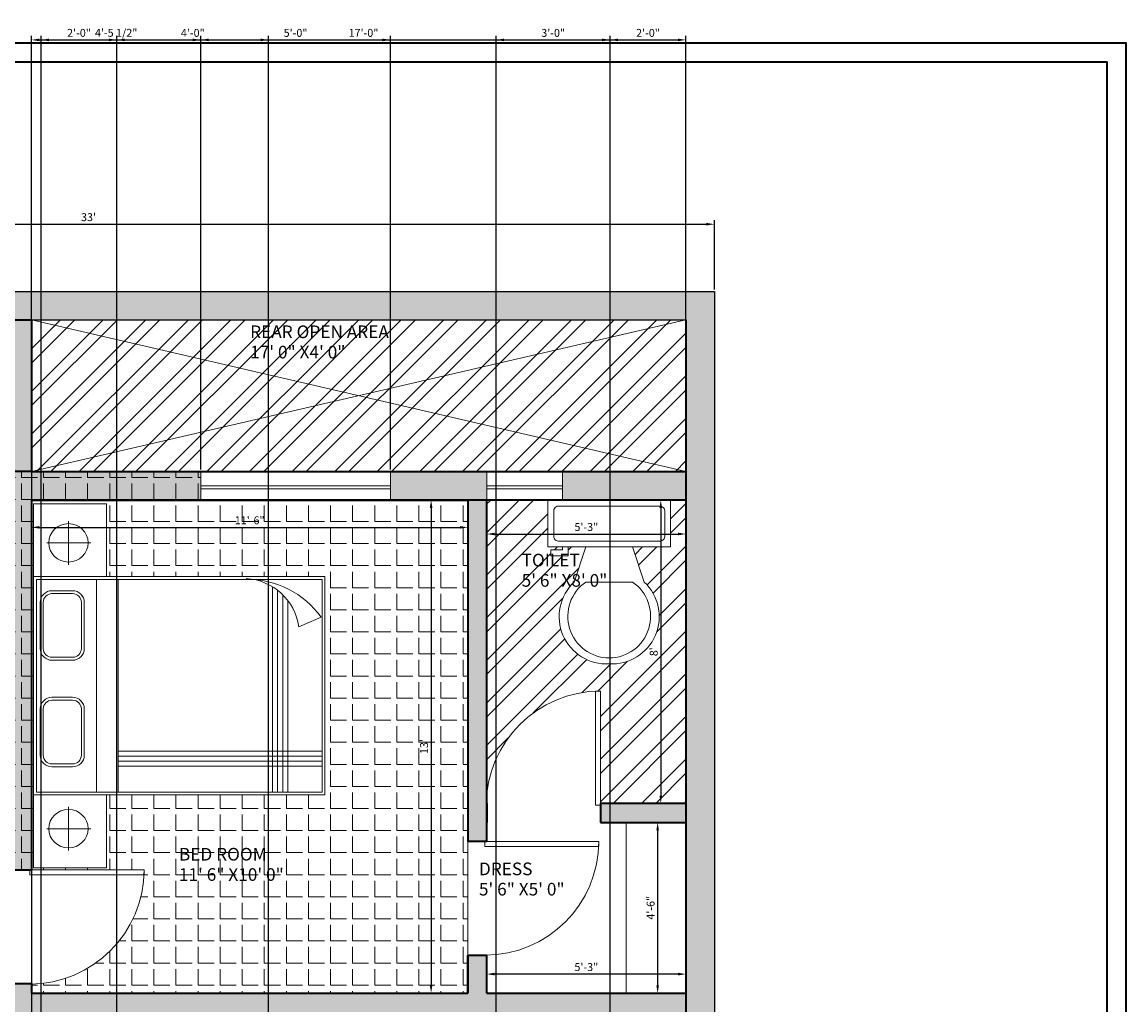
# Model space of a CAD drawing. Units: inches. Extents: x 2004 to 2661, y 1548 to 2351.
# Tile 5 of 5: x 2312 to 2661, y 2040 to 2351. Entities that reach past the tile are written whole.
import ezdxf

# ---------------------------------------------------------------- set-up
doc = ezdxf.new("R2010")
doc.units = ezdxf.units.IN
for name, color, linetype, lineweight in [('A-ANNO-DIMS', 2, 'Continuous', 18), ('A-ANNO-TTLB', 7, 'Continuous', 35), ('A-AREA-IDEN', 7, 'Continuous', 18), ('A-DOOR', 3, 'Continuous', 18), ('A-FLOR-CASE', 8, 'Continuous', 18), ('A-FLOR-FIXT', 9, 'Continuous', 18), ('A-FURN', 8, 'Continuous', 18), ('A-GLAZ', 4, 'Continuous', 18), ('A-SITE', 8, 'Continuous', 13), ('A-WALL', 7, 'Continuous', 35), ('C-PROP', 7, 'Continuous', 25)]:
    doc.layers.add(name, color=color, linetype=linetype, lineweight=lineweight)
doc.layers.add('A-FLOR-PATT', color=18, linetype='Continuous', lineweight=13, true_color=0x000000)
doc.layers.add('A-WALL-PATT', color=18, linetype='Continuous', lineweight=13, true_color=0x000000)
doc.styles.get("Standard").update_dxf_attribs({"font": 'arial.ttf'})
doc.dimstyles.new('Copy of ISO-25', dxfattribs={"dimtxt": 2.5, "dimasz": 2.5, "dimexe": 1.25, "dimexo": 0.625, "dimtad": 1, "dimlunit": 4, "dimtxsty": 'Standard', "dimcen": 2.5, "dimadec": 0, "dimazin": 0, "dimtfac": 1, "dimtmove": 0, "dimatfit": 3, "dimfxl": 1, "dimarcsym": 0})

# ---------------------------------------------------------------- blocks, each defined once
blk = doc.blocks.new('*D1')
at = {"layer": 'A-ANNO-DIMS', "color": 0, "lineweight": -2, "transparency": 16777216}
for p, q in [((2135.26, 2266.72), (2135.26, 2288.6)), ((2137.76, 2287.35), (2528.76, 2287.35)), ((2531.26, 2266.72), (2531.26, 2288.6))]:
    blk.add_line(p, q, dxfattribs=at)
at = {"layer": 'A-ANNO-DIMS', "color": 0, "transparency": 16777216}
for points in [[(2137.76, 2287.77), (2137.76, 2286.93), (2135.26, 2287.35)], [(2528.76, 2287.77), (2528.76, 2286.93), (2531.26, 2287.35)]]:
    blk.add_solid(points, dxfattribs=at)
at = {"layer": 'Defpoints', "color": 0, "transparency": 16777216}
for p in [(2531.26, 2287.35), (2135.26, 2266.09), (2531.26, 2266.09)]:
    blk.add_point(p, dxfattribs=at)
at = {"layer": 'A-ANNO-DIMS', "color": 0, "transparency": 16777216, "insert": (2333.26, 2289.25), "char_height": 2.5, "attachment_point": 5}
blk.add_mtext("33'", dxfattribs=at)
blk = doc.blocks.new('A$C057D194F')
for p, q in [((0, 1.5, -0.1688), (0, 2, -0.1688)), ((0, 2, -0.1688), (0.5, 2, -0.1688)), ((0.5, 2, -0.1688), (0.5, 0, -0.1688)), ((2, 2, -0.1688), (0.5, 2, -0.1688)), ((1.98, 1.98, -0.1688), (0.52, 1.98, -0.1688)), ((0.52, 1.98, -0.1688), (0.52, 0.02, -0.1688)), ((1.98, 0.02, -0.1688), (1.98, 1.98, -0.1688)), ((2, 0, -0.1688), (2, 2, -0.1688)), ((2.5, 2, -0.1688), (2, 2, -0.1688)), ((2.5, 1.5, -0.1688), (2.5, 2, -0.1688)), ((0.2687, 1.9081, -0.1688), (0.2687, 1.761, -0.1688)), ((0.2687, 1.6081, -0.1688), (0.2687, 1.9081, -0.1688)), ((1.0907, 1.9539, -0.1688), (0.7735, 1.9539, -0.1688)), ((1.0907, 1.9339, -0.1688), (0.7735, 1.9339, -0.1688)), ((1.8224, 1.9539, -0.1688), (1.5052, 1.9539, -0.1688)), ((1.8224, 1.9339, -0.1688), (1.5052, 1.9339, -0.1688)), ((2.2313, 1.9081, -0.1688), (2.2313, 1.761, -0.1688)), ((2.2313, 1.6081, -0.1688), (2.2313, 1.9081, -0.1688)), ((0.6935, 1.8739, -0.1688), (0.6935, 1.7322, -0.1688)), ((0.7135, 1.8739, -0.1688), (0.7135, 1.7322, -0.1688)), ((1.1507, 1.7322, -0.1688), (1.1507, 1.8739, -0.1688)), ((1.1707, 1.7322, -0.1688), (1.1707, 1.8739, -0.1688)), ((1.4252, 1.8739, -0.1688), (1.4252, 1.7322, -0.1688)), ((1.4452, 1.8739, -0.1688), (1.4452, 1.7322, -0.1688)), ((1.8824, 1.7322, -0.1688), (1.8824, 1.8739, -0.1688)), ((1.9024, 1.7322, -0.1688), (1.9024, 1.8739, -0.1688)), ((0.4194, 1.761, -0.1688), (0.1194, 1.761, -0.1688)), ((0.2687, 1.761, -0.1688), (0.4194, 1.761, -0.1688)), ((0.2687, 1.761, -0.1688), (0.2687, 1.6081, -0.1688)), ((2.0806, 1.761, -0.1688), (2.3806, 1.761, -0.1688)), ((2.2313, 1.761, -0.1688), (2.0806, 1.761, -0.1688)), ((2.2313, 1.761, -0.1688), (2.2313, 1.6081, -0.1688)), ((0.7735, 1.6722, -0.1688), (1.0907, 1.6722, -0.1688)), ((1.5052, 1.6722, -0.1688), (1.8224, 1.6722, -0.1688)), ((0.7735, 1.6522, -0.1688), (1.0907, 1.6522, -0.1688)), ((1.5052, 1.6522, -0.1688), (1.8224, 1.6522, -0.1688)), ((1.98, 1.5693, -0.1688), (0.52, 1.5693, -0.1688)), ((0.5, 1.5, -0.1688), (0, 1.5, -0.1688)), ((2, 1.5, -0.1688), (2.5, 1.5, -0.1688)), ((1.98, 1.4193, -0.1688), (0.52, 1.4193, -0.1688)), ((0.6969, 0.02, -0.1688), (0.6969, 1.4193, -0.1688)), ((0.7319, 0.02, -0.1688), (0.7319, 1.4193, -0.1688)), ((0.7669, 0.02, -0.1688), (0.7669, 1.4193, -0.1688)), ((0.8019, 0.02, -0.1688), (0.8019, 1.4193, -0.1688)), ((0.52, 0.3595, -0.1688), (1.9292, 0.3595, -0.1688)), ((0.52, 0.3245, -0.1688), (1.905, 0.3245, -0.1688)), ((0.52, 0.2895, -0.1688), (1.8742, 0.2895, -0.1688)), ((0.52, 0.2545, -0.1688), (1.8344, 0.2545, -0.1688)), ((1.6548, 0.1789, -0.1688), (1.7198, 0.0251, -0.1688)), ((0.52, 0.02, -0.1688), (1.98, 0.02, -0.1688)), ((0.5, 0, -0.1688), (2, 0, -0.1688))]:
    blk.add_line(p, q)
for centre, radius, start, end in [((0.7735, 1.8739, -0.1688), 0.08, 90, 180), ((0.7735, 1.8739, -0.1688), 0.06, 90, 180), ((1.0907, 1.8739, -0.1688), 0.08, 0, 90), ((1.0907, 1.8739, -0.1688), 0.06, 0, 90), ((1.5052, 1.8739, -0.1688), 0.08, 90, 180), ((1.5052, 1.8739, -0.1688), 0.06, 90, 180), ((1.8224, 1.8739, -0.1688), 0.08, 0, 90), ((1.8224, 1.8739, -0.1688), 0.06, 0, 90), ((0.7735, 1.7322, -0.1688), 0.08, 180, 270), ((0.7735, 1.7322, -0.1688), 0.06, 180, 270), ((1.0907, 1.7322, -0.1688), 0.08, 270, 0), ((1.0907, 1.7322, -0.1688), 0.06, 270, 0), ((1.5052, 1.7322, -0.1688), 0.08, 180, 270), ((1.5052, 1.7322, -0.1688), 0.06, 180, 270), ((1.8224, 1.7322, -0.1688), 0.08, 270, 0), ((1.8224, 1.7322, -0.1688), 0.06, 270, 0), ((1.5992, 0.5623, -0.1688), 0.3874, 278.2518, 356.6808), ((1.363, 0.5286, -0.1688), 0.6171, 305.32946, 1.04595)]:
    blk.add_arc(centre, radius, start, end)
blk.add_ellipse((0.2687, 1.761, -0.1688), major_axis=(0, -0.1351), ratio=0.975448)
at = {"extrusion": (0, 0, -1)}
blk.add_ellipse((2.2313, 1.761, -0.1688), major_axis=(0, 0.1351), ratio=0.975448, dxfattribs=at)
for p in [(0.2687, 1.761, -0.1688), (2.2313, 1.761, -0.1688)]:
    blk.add_point(p)
blk = doc.blocks.new('*U7')
for p, q in [((-40, 0), (-40, 6)), ((0, 0), (0, 6))]:
    blk.add_line(p, q)
blk.add_lwpolyline([(0, 0), (0, -40), (-1.75, -40), (-1.75, 0)], close=True)
blk.add_arc((0, 0), 40, 180, 270)
blk = doc.blocks.new('*U6')
for p, q in [((0, 0), (0, -6)), ((-40, 0), (-40, -6))]:
    blk.add_line(p, q)
blk.add_lwpolyline([(0, 0), (0, 40), (-1.75, 40), (-1.75, 0)], close=True)
blk.add_arc((0, 0), 40, 90, 180)
blk = doc.blocks.new('*U10')
for p, q in [((241.3, -152.4), (241.3, -50.8)), ((-254, -215.9), (-203.2, -215.9)), ((-254, -241.3), (-254, -215.9)), ((-203.2, -215.9), (-203.2, -203.2)), ((-177.8, -203.2), (-177.8, -241.3)), ((-101.6, -203.2), (-152.4, -355.6)), ((101.6, -203.2), (152.4, -355.6)), ((-177.8, -241.3), (-254, -241.3)), ((101.6, -355.6), (-101.6, -355.6))]:
    blk.add_line(p, q)
blk.add_lwpolyline([(266.7, -203.2), (266.7, 0), (-266.7, 0), (-266.7, -203.2)], close=True)
for points in [[(215.9, -25.4), (-215.9, -25.4)], [(-241.3, -50.8), (-241.3, -152.4)], [(-215.9, -177.8), (215.9, -177.8)]]:
    blk.add_lwpolyline(points)
for centre, radius, start, end in [((-219.075, -47.625), 22.45064, 81.8699, 188.1301), ((219.075, -47.625), 22.45064, 351.8699, 98.1301), ((-219.075, -155.575), 22.45064, 171.869898, 278.1301), ((219.075, -155.575), 22.45064, 261.8699, 8.1301), ((-12.12088, -505.93752), 205.61935, 133.01722, 273.38), ((0.94996, -504.77674), 181.02486, 124.50543, 269.7), ((-0.94742, -504.77674), 181.02486, 270.3, 55.4946), ((12.12342, -505.93752), 205.61935, 266.62, 46.9828)]:
    blk.add_arc(centre, radius, start, end)
blk = doc.blocks.new('*D17')
at = {"layer": 'A-ANNO-DIMS', "color": 0, "lineweight": -2, "transparency": 16777216}
for p, q in [((2315.26, 2199.47), (2315.26, 2190.19)), ((2453.26, 2199.47), (2453.26, 2190.19)), ((2317.76, 2191.44), (2450.76, 2191.44))]:
    blk.add_line(p, q, dxfattribs=at)
at = {"layer": 'A-ANNO-DIMS', "color": 0, "transparency": 16777216}
for points in [[(2317.76, 2191.86), (2317.76, 2191.03), (2315.26, 2191.44)], [(2450.76, 2191.86), (2450.76, 2191.03), (2453.26, 2191.44)]]:
    blk.add_solid(points, dxfattribs=at)
at = {"layer": 'Defpoints', "color": 0, "transparency": 16777216}
for p in [(2315.26, 2200.09), (2453.26, 2200.09), (2453.26, 2191.44)]:
    blk.add_point(p, dxfattribs=at)
at = {"layer": 'A-ANNO-DIMS', "color": 0, "transparency": 16777216, "insert": (2384.26, 2193.34), "char_height": 2.5, "attachment_point": 5}
blk.add_mtext('11\'-6"', dxfattribs=at)
blk = doc.blocks.new('*D18')
at = {"layer": 'A-ANNO-DIMS', "color": 0, "lineweight": -2, "transparency": 16777216}
for p, q in [((2452.63, 2200.09), (2440.4, 2200.09)), ((2441.65, 2197.59), (2441.65, 2046.59)), ((2452.63, 2044.09), (2440.4, 2044.09))]:
    blk.add_line(p, q, dxfattribs=at)
at = {"layer": 'A-ANNO-DIMS', "color": 0, "transparency": 16777216}
for points in [[(2441.23, 2197.59), (2442.06, 2197.59), (2441.65, 2200.09)], [(2441.23, 2046.59), (2442.06, 2046.59), (2441.65, 2044.09)]]:
    blk.add_solid(points, dxfattribs=at)
at = {"layer": 'Defpoints', "color": 0, "transparency": 16777216}
for p in [(2453.26, 2200.09), (2441.65, 2044.09), (2453.26, 2044.09)]:
    blk.add_point(p, dxfattribs=at)
at = {"layer": 'A-ANNO-DIMS', "color": 0, "transparency": 16777216, "insert": (2439.74, 2122.09), "char_height": 2.5, "attachment_point": 5, "rotation": 90}
blk.add_mtext("13'", dxfattribs=at)
blk = doc.blocks.new('*D19')
at = {"layer": 'A-ANNO-DIMS', "color": 0, "lineweight": -2, "transparency": 16777216}
for p, q in [((2459.26, 2199.47), (2459.26, 2188.08)), ((2522.26, 2199.47), (2522.26, 2188.08)), ((2461.76, 2189.33), (2519.76, 2189.33))]:
    blk.add_line(p, q, dxfattribs=at)
at = {"layer": 'A-ANNO-DIMS', "color": 0, "transparency": 16777216}
for points in [[(2461.76, 2189.75), (2461.76, 2188.91), (2459.26, 2189.33)], [(2519.76, 2189.75), (2519.76, 2188.91), (2522.26, 2189.33)]]:
    blk.add_solid(points, dxfattribs=at)
at = {"layer": 'Defpoints', "color": 0, "transparency": 16777216}
for p in [(2459.26, 2200.09), (2522.26, 2200.09), (2522.26, 2189.33)]:
    blk.add_point(p, dxfattribs=at)
at = {"layer": 'A-ANNO-DIMS', "color": 0, "transparency": 16777216, "insert": (2490.76, 2191.23), "char_height": 2.5, "attachment_point": 5}
blk.add_mtext('5\'-3"', dxfattribs=at)
blk = doc.blocks.new('*D20')
at = {"layer": 'A-ANNO-DIMS', "color": 0, "lineweight": -2, "transparency": 16777216}
for p, q in [((2521.63, 2200.09), (2513.05, 2200.09)), ((2514.3, 2197.59), (2514.3, 2106.59)), ((2521.63, 2104.09), (2513.05, 2104.09))]:
    blk.add_line(p, q, dxfattribs=at)
at = {"layer": 'A-ANNO-DIMS', "color": 0, "transparency": 16777216}
for points in [[(2513.89, 2197.59), (2514.72, 2197.59), (2514.3, 2200.09)], [(2513.89, 2106.59), (2514.72, 2106.59), (2514.3, 2104.09)]]:
    blk.add_solid(points, dxfattribs=at)
at = {"layer": 'Defpoints', "color": 0, "transparency": 16777216}
for p in [(2522.26, 2200.09), (2514.3, 2104.09), (2522.26, 2104.09)]:
    blk.add_point(p, dxfattribs=at)
at = {"layer": 'A-ANNO-DIMS', "color": 0, "transparency": 16777216, "insert": (2512.4, 2152.09), "char_height": 2.5, "attachment_point": 5, "rotation": 90}
blk.add_mtext("8'", dxfattribs=at)
blk = doc.blocks.new('*D21')
at = {"layer": 'A-ANNO-DIMS', "color": 0, "lineweight": -2, "transparency": 16777216}
for p, q in [((2459.26, 2044.72), (2459.26, 2051.34)), ((2519.76, 2050.09), (2461.76, 2050.09)), ((2522.26, 2044.72), (2522.26, 2051.34))]:
    blk.add_line(p, q, dxfattribs=at)
at = {"layer": 'A-ANNO-DIMS', "color": 0, "transparency": 16777216}
for points in [[(2461.76, 2050.51), (2461.76, 2049.68), (2459.26, 2050.09)], [(2519.76, 2050.51), (2519.76, 2049.68), (2522.26, 2050.09)]]:
    blk.add_solid(points, dxfattribs=at)
at = {"layer": 'Defpoints', "color": 0, "transparency": 16777216}
for p in [(2459.26, 2050.09), (2459.26, 2044.09), (2522.26, 2044.09)]:
    blk.add_point(p, dxfattribs=at)
at = {"layer": 'A-ANNO-DIMS', "color": 0, "transparency": 16777216, "insert": (2490.76, 2051.99), "char_height": 2.5, "attachment_point": 5}
blk.add_mtext('5\'-3"', dxfattribs=at)
blk = doc.blocks.new('*D22')
at = {"layer": 'A-ANNO-DIMS', "color": 0, "lineweight": -2, "transparency": 16777216}
for p, q in [((2521.63, 2098.09), (2512.06, 2098.09)), ((2513.31, 2095.59), (2513.31, 2046.59)), ((2521.63, 2044.09), (2512.06, 2044.09))]:
    blk.add_line(p, q, dxfattribs=at)
at = {"layer": 'A-ANNO-DIMS', "color": 0, "transparency": 16777216}
for points in [[(2512.89, 2095.59), (2513.73, 2095.59), (2513.31, 2098.09)], [(2512.89, 2046.59), (2513.73, 2046.59), (2513.31, 2044.09)]]:
    blk.add_solid(points, dxfattribs=at)
at = {"layer": 'Defpoints', "color": 0, "transparency": 16777216}
for p in [(2522.26, 2098.09), (2513.31, 2044.09), (2522.26, 2044.09)]:
    blk.add_point(p, dxfattribs=at)
at = {"layer": 'A-ANNO-DIMS', "color": 0, "transparency": 16777216, "insert": (2511.41, 2071.09), "char_height": 2.5, "attachment_point": 5, "rotation": 90}
blk.add_mtext('4\'-6"', dxfattribs=at)
blk = doc.blocks.new('WINDOW-PANE-24IN')
for p, q in [((0, 1), (24, 1)), ((0, 0), (24, 0))]:
    blk.add_line(p, q)
blk = doc.blocks.new('*D41')
at = {"layer": 'A-ANNO-DIMS', "color": 0, "lineweight": -2, "transparency": 16777216}
for p, q in [((2318.26, 1675.72), (2318.26, 2346.91)), ((2522.26, 1675.72), (2522.26, 2346.91)), ((2320.76, 2345.66), (2519.76, 2345.66))]:
    blk.add_line(p, q, dxfattribs=at)
at = {"layer": 'A-ANNO-DIMS', "color": 0, "transparency": 16777216}
for points in [[(2320.76, 2346.07), (2320.76, 2345.24), (2318.26, 2345.66)], [(2519.76, 2346.07), (2519.76, 2345.24), (2522.26, 2345.66)]]:
    blk.add_solid(points, dxfattribs=at)
at = {"layer": 'Defpoints', "color": 0, "transparency": 16777216}
for p in [(2522.26, 2345.66), (2318.26, 1675.09), (2522.26, 1675.09)]:
    blk.add_point(p, dxfattribs=at)
at = {"layer": 'A-ANNO-DIMS', "color": 0, "transparency": 16777216, "insert": (2420.26, 2347.56), "char_height": 2.5, "attachment_point": 5}
blk.add_mtext('17\'-0"', dxfattribs=at)
blk = doc.blocks.new('*D42')
at = {"layer": 'A-ANNO-DIMS', "color": 0, "lineweight": -2, "transparency": 16777216}
for p, q in [((2315.26, 2256.47), (2315.26, 1630.09)), ((2522.26, 2256.47), (2522.26, 1630.09)), ((2317.76, 1631.34), (2519.76, 1631.34))]:
    blk.add_line(p, q, dxfattribs=at)
at = {"layer": 'A-ANNO-DIMS', "color": 0, "transparency": 16777216}
for points in [[(2317.76, 1631.76), (2317.76, 1630.93), (2315.26, 1631.34)], [(2519.76, 1631.76), (2519.76, 1630.93), (2522.26, 1631.34)]]:
    blk.add_solid(points, dxfattribs=at)
at = {"layer": 'Defpoints', "color": 0, "transparency": 16777216}
for p in [(2315.26, 2257.09), (2522.26, 2257.09), (2522.26, 1631.34)]:
    blk.add_point(p, dxfattribs=at)
at = {"layer": 'A-ANNO-DIMS', "color": 0, "transparency": 16777216, "insert": (2418.76, 1633.24), "char_height": 2.5, "attachment_point": 5}
blk.add_mtext('17\'-3"', dxfattribs=at)
blk = doc.blocks.new('*D48')
at = {"layer": 'A-ANNO-DIMS', "color": 0, "lineweight": -2, "transparency": 16777216}
for p, q in [((2315.26, 2209.72), (2315.26, 2346.91)), ((2368.77, 2209.72), (2368.77, 2346.91)), ((2317.76, 2345.66), (2366.27, 2345.66))]:
    blk.add_line(p, q, dxfattribs=at)
at = {"layer": 'A-ANNO-DIMS', "color": 0, "transparency": 16777216}
for points in [[(2317.76, 2346.07), (2317.76, 2345.24), (2315.26, 2345.66)], [(2366.27, 2346.07), (2366.27, 2345.24), (2368.77, 2345.66)]]:
    blk.add_solid(points, dxfattribs=at)
at = {"layer": 'Defpoints', "color": 0, "transparency": 16777216}
for p in [(2368.77, 2345.66), (2315.26, 2209.09), (2368.77, 2209.09)]:
    blk.add_point(p, dxfattribs=at)
at = {"layer": 'A-ANNO-DIMS', "color": 0, "transparency": 16777216, "insert": (2342.01, 2347.58), "char_height": 2.5, "attachment_point": 5}
blk.add_mtext('4\'-5 1/2"', dxfattribs=at)
blk = doc.blocks.new('*D49')
at = {"layer": 'A-ANNO-DIMS', "color": 0, "lineweight": -2, "transparency": 16777216}
for p, q in [((2368.77, 2209.72), (2368.77, 2346.91)), ((2428.77, 2209.72), (2428.77, 2346.91)), ((2371.27, 2345.66), (2426.27, 2345.66))]:
    blk.add_line(p, q, dxfattribs=at)
at = {"layer": 'A-ANNO-DIMS', "color": 0, "transparency": 16777216}
for points in [[(2371.27, 2346.07), (2371.27, 2345.24), (2368.77, 2345.66)], [(2426.27, 2346.07), (2426.27, 2345.24), (2428.77, 2345.66)]]:
    blk.add_solid(points, dxfattribs=at)
at = {"layer": 'Defpoints', "color": 0, "transparency": 16777216}
for p in [(2428.77, 2345.66), (2368.77, 2209.09), (2428.77, 2209.09)]:
    blk.add_point(p, dxfattribs=at)
at = {"layer": 'A-ANNO-DIMS', "color": 0, "transparency": 16777216, "insert": (2398.77, 2347.56), "char_height": 2.5, "attachment_point": 5}
blk.add_mtext('5\'-0"', dxfattribs=at)
blk = doc.blocks.new('*D50')
at = {"layer": 'A-ANNO-DIMS', "color": 0, "lineweight": -2, "transparency": 16777216}
for p, q in [((2318.26, 1762.72), (2318.26, 2346.91)), ((2342.26, 1762.72), (2342.26, 2346.91)), ((2320.76, 2345.66), (2339.76, 2345.66))]:
    blk.add_line(p, q, dxfattribs=at)
at = {"layer": 'A-ANNO-DIMS', "color": 0, "transparency": 16777216}
for points in [[(2320.76, 2346.07), (2320.76, 2345.24), (2318.26, 2345.66)], [(2339.76, 2346.07), (2339.76, 2345.24), (2342.26, 2345.66)]]:
    blk.add_solid(points, dxfattribs=at)
at = {"layer": 'Defpoints', "color": 0, "transparency": 16777216}
for p in [(2342.26, 2345.66), (2318.26, 1762.09), (2342.26, 1762.09)]:
    blk.add_point(p, dxfattribs=at)
at = {"layer": 'A-ANNO-DIMS', "color": 0, "transparency": 16777216, "insert": (2330.26, 2347.56), "char_height": 2.5, "attachment_point": 5}
blk.add_mtext('2\'-0"', dxfattribs=at)
blk = doc.blocks.new('*D51')
at = {"layer": 'A-ANNO-DIMS', "color": 0, "lineweight": -2, "transparency": 16777216}
for p, q in [((2342.26, 1762.72), (2342.26, 2346.91)), ((2390.26, 1762.72), (2390.26, 2346.91)), ((2344.76, 2345.66), (2387.76, 2345.66))]:
    blk.add_line(p, q, dxfattribs=at)
at = {"layer": 'A-ANNO-DIMS', "color": 0, "transparency": 16777216}
for points in [[(2344.76, 2346.07), (2344.76, 2345.24), (2342.26, 2345.66)], [(2387.76, 2346.07), (2387.76, 2345.24), (2390.26, 2345.66)]]:
    blk.add_solid(points, dxfattribs=at)
at = {"layer": 'Defpoints', "color": 0, "transparency": 16777216}
for p in [(2390.26, 2345.66), (2342.26, 1762.09), (2390.26, 1762.09)]:
    blk.add_point(p, dxfattribs=at)
at = {"layer": 'A-ANNO-DIMS', "color": 0, "transparency": 16777216, "insert": (2366.26, 2347.56), "char_height": 2.5, "attachment_point": 5}
blk.add_mtext('4\'-0"', dxfattribs=at)
blk = doc.blocks.new('*D52')
at = {"layer": 'A-ANNO-DIMS', "color": 0, "lineweight": -2, "transparency": 16777216}
for p, q in [((2462.26, 1762.72), (2462.26, 2346.91)), ((2498.26, 1762.72), (2498.26, 2346.91)), ((2464.76, 2345.66), (2495.76, 2345.66))]:
    blk.add_line(p, q, dxfattribs=at)
at = {"layer": 'A-ANNO-DIMS', "color": 0, "transparency": 16777216}
for points in [[(2464.76, 2346.07), (2464.76, 2345.24), (2462.26, 2345.66)], [(2495.76, 2346.07), (2495.76, 2345.24), (2498.26, 2345.66)]]:
    blk.add_solid(points, dxfattribs=at)
at = {"layer": 'Defpoints', "color": 0, "transparency": 16777216}
for p in [(2498.26, 2345.66), (2462.26, 1762.09), (2498.26, 1762.09)]:
    blk.add_point(p, dxfattribs=at)
at = {"layer": 'A-ANNO-DIMS', "color": 0, "transparency": 16777216, "insert": (2480.26, 2347.56), "char_height": 2.5, "attachment_point": 5}
blk.add_mtext('3\'-0"', dxfattribs=at)
blk = doc.blocks.new('*D53')
at = {"layer": 'A-ANNO-DIMS', "color": 0, "lineweight": -2, "transparency": 16777216}
for p, q in [((2498.26, 1762.72), (2498.26, 2346.91)), ((2522.26, 1762.72), (2522.26, 2346.91)), ((2500.76, 2345.66), (2519.76, 2345.66))]:
    blk.add_line(p, q, dxfattribs=at)
at = {"layer": 'A-ANNO-DIMS', "color": 0, "transparency": 16777216}
for points in [[(2500.76, 2346.07), (2500.76, 2345.24), (2498.26, 2345.66)], [(2519.76, 2346.07), (2519.76, 2345.24), (2522.26, 2345.66)]]:
    blk.add_solid(points, dxfattribs=at)
at = {"layer": 'Defpoints', "color": 0, "transparency": 16777216}
for p in [(2522.26, 2345.66), (2498.26, 1762.09), (2522.26, 1762.09)]:
    blk.add_point(p, dxfattribs=at)
at = {"layer": 'A-ANNO-DIMS', "color": 0, "transparency": 16777216, "insert": (2510.26, 2347.56), "char_height": 2.5, "attachment_point": 5}
blk.add_mtext('2\'-0"', dxfattribs=at)

msp = doc.modelspace()

# ---------------------------------------------------------------- hatches: boundary and pattern name
at = {"layer": 'A-FLOR-PATT'}
h = msp.add_hatch(dxfattribs=at)
h.set_pattern_fill('ANSI32', color=256)
h.paths.add_polyline_path([(2522.257, 2257.093), (2466.833, 2257.093), (2315.257, 2257.093), (2418.757, 2233.093)])
h.paths.add_polyline_path([(2418.757, 2233.093), (2315.257, 2257.093), (2315.257, 2209.093)])
h.paths.add_polyline_path([(2418.757, 2233.093), (2315.257, 2209.093), (2522.257, 2209.093)])
h.paths.add_polyline_path([(2522.257, 2257.093), (2418.757, 2233.093), (2522.257, 2209.093)])
h.paths.add_polyline_path([(2522.257, 1753.093), (2318.257, 1753.093), (2318.257, 1675.093), (2522.257, 1675.093)])
h.paths.add_polyline_path([(2210.267, 2081.517), (2210.233, 2081.517), (2210.233, 2083.093), (2246.257, 2083.093), (2246.257, 2119.093), (2144.257, 2119.093), (2144.257, 2047.093), (2244.938, 2047.093, -0.390864)])
h.paths.add_polyline_path([(2171.613, 2077.721), (2161.069, 2080.96), (2161.193, 2075.729), (2163.808, 2075.791), (2163.932, 2070.56), (2162.189, 2070.519), (2162.106, 2074.006), (2161.234, 2073.986), (2161.338, 2069.627), (2147.389, 2069.296), (2146.521, 2105.911), (2160.469, 2106.241), (2160.738, 2094.908), (2171.117, 2098.643, -0.7025712), (2195.775, 2088.761, -0.7025621)], flags=16)
h.paths.add_polyline_path([(2171.53, 2081.208), (2171.2, 2095.156, -0.7345333), (2194.031, 2088.72, -0.7345297)], flags=0)
h.paths.add_polyline_path([(2158.245, 2071.298), (2150.835, 2071.122, -0.4142136), (2149.061, 2072.388), (2148.347, 2102.465, -0.4142136), (2149.614, 2104.239), (2157.024, 2104.415, -0.4142136), (2158.798, 2103.149), (2159.512, 2073.072, -0.4142136)], flags=0)
h.paths.add_polyline_path([(2522.257, 2200.093), (2517.397, 2200.093), (2517.397, 2185.232), (2505.384, 2185.232), (2509.08, 2174.143, -0.7025712), (2497.991, 2148.268, -0.7025621), (2486.902, 2174.142), (2490.599, 2185.232), (2485.054, 2185.232), (2485.054, 2182.459), (2479.509, 2182.459), (2479.509, 2184.307), (2483.206, 2184.307), (2483.206, 2185.232), (2478.585, 2185.232), (2478.585, 2200.093), (2459.257, 2200.093), (2459.257, 2106.686, -0.3761573), (2493.676, 2139.619), (2493.676, 2139.653), (2495.257, 2139.653), (2495.257, 2104.093), (2522.257, 2104.093)])
h.paths.add_polyline_path([(2349.854, 1719.146), (2381.921, 1719.146), (2381.921, 1725.273), (2349.854, 1725.273)], flags=24)
h.paths.add_polyline_path([(2349.84, 1725.558), (2388.851, 1725.558), (2388.851, 1731.767), (2349.84, 1731.767)], flags=24)
h.paths.add_polyline_path([(2152.908, 2086.679), (2181.867, 2086.679), (2181.867, 2092.806), (2152.908, 2092.806)], flags=8)
h.paths.add_polyline_path([(2152.895, 2093.091), (2174.525, 2093.091), (2174.525, 2099.3), (2152.895, 2099.3)], flags=8)
h.paths.add_polyline_path([(2515.001, 2150.174), (2515.001, 2154.033), (2509.85, 2154.033), (2509.85, 2150.174)], flags=24)
h.paths.add_polyline_path([(2469.272, 2171.563), (2498.231, 2171.563), (2498.231, 2177.69), (2469.272, 2177.69)], flags=24)
h.paths.add_polyline_path([(2469.258, 2177.975), (2490.888, 2177.975), (2490.888, 2184.184), (2469.258, 2184.184)], flags=24)
h = msp.add_hatch(dxfattribs=at)
h.set_pattern_fill('ANGLE', color=256)
h.set_pattern_definition([(0, (0, 0), (0, 6.985), [5.08, -1.905]), (90, (0, 0), (-6.985, 4e-16), [5.08, -1.905])])
h.paths.add_polyline_path([(2453.257, 2092.093), (2453.257, 2200.093), (2368.773, 2200.093), (2368.773, 2209.093), (2315.257, 2209.093), (2309.257, 2209.093), (2309.257, 2119.093), (2309.257, 2083.093), (2315.257, 2083.093), (2350.837, 2083.093), (2350.837, 2081.511), (2350.802, 2081.511, -0.3968312), (2315.257, 2046.941), (2315.257, 2044.093), (2453.257, 2044.093), (2453.257, 2056.093)])
h.paths.add_polyline_path([(2338.94, 2106.763), (2338.94, 2083.722), (2315.9, 2083.722), (2315.9, 2106.763), (2315.9, 2175.884), (2315.9, 2198.924), (2338.94, 2198.924), (2338.94, 2175.884), (2408.062, 2175.884), (2408.062, 2106.763)], flags=16)
h.paths.add_polyline_path([(2316.822, 2107.684), (2316.822, 2174.962), (2383.185, 2174.962, -0.0091279), (2384.223, 2174.962), (2407.14, 2174.962), (2407.14, 2107.684)], flags=0)
h.paths.add_polyline_path([(2342.657, 2115.838), (2342.657, 2120.677), (2391.497, 2120.677), (2391.497, 2172.623, -0.0921038), (2396.336, 2168.251), (2396.336, 2115.838)], flags=0)
h.paths.add_polyline_path([(2393.11, 2119.064), (2394.723, 2119.064), (2394.723, 2117.451), (2393.11, 2117.451)], flags=0)
edge = h.paths.add_edge_path(flags=0)
edge.add_ellipse((2326.912, 2096.106), major_axis=(-6.224, 0), ratio=0.9754478, start_angle=450, end_angle=540, ccw=False)
edge.add_ellipse((2326.912, 2096.106), major_axis=(-6.224, 0), ratio=0.9754478, start_angle=360, end_angle=450, ccw=False)
edge.add_ellipse((2326.912, 2096.106), major_axis=(-6.224, 0), ratio=0.9754478, start_angle=270, end_angle=360, ccw=False)
edge.add_ellipse((2326.912, 2096.106), major_axis=(-6.224, 0), ratio=0.9754478, start_angle=180, end_angle=270, ccw=False)
h.paths.add_polyline_path([(2328.241, 2115.678), (2321.709, 2115.678, -0.4142136), (2318.023, 2119.364), (2318.023, 2133.984, -0.4142136), (2321.709, 2137.671), (2328.241, 2137.671, -0.4142136), (2331.928, 2133.984), (2331.928, 2119.364, -0.4142136)], flags=0)
h.paths.add_polyline_path([(2328.241, 2116.599), (2321.709, 2116.599, -0.4142136), (2318.945, 2119.364), (2318.945, 2133.984, -0.4142136), (2321.709, 2136.749), (2328.241, 2136.749, -0.4142136), (2331.006, 2133.984), (2331.006, 2119.364, -0.4142136)], flags=0)
h.paths.add_polyline_path([(2328.241, 2149.395), (2321.709, 2149.395, -0.4142136), (2318.023, 2153.081), (2318.023, 2167.701, -0.4142136), (2321.709, 2171.388), (2328.241, 2171.388, -0.4142136), (2331.928, 2167.701), (2331.928, 2153.081, -0.4142136)], flags=0)
h.paths.add_polyline_path([(2328.241, 2150.316), (2321.709, 2150.316, -0.4142136), (2318.945, 2153.081), (2318.945, 2167.701, -0.4142136), (2321.709, 2170.466), (2328.241, 2170.466, -0.4142136), (2331.006, 2167.701), (2331.006, 2153.081, -0.4142136)], flags=0)
edge = h.paths.add_edge_path(flags=0)
edge.add_ellipse((2326.912, 2186.54), major_axis=(-6.224, 0), ratio=0.9754478, start_angle=0, end_angle=90, ccw=False)
edge.add_ellipse((2326.912, 2186.54), major_axis=(-6.224, 0), ratio=0.9754478, start_angle=270, end_angle=360, ccw=False)
edge.add_ellipse((2326.912, 2186.54), major_axis=(-6.224, 0), ratio=0.9754478, start_angle=180, end_angle=270, ccw=False)
edge.add_ellipse((2326.912, 2186.54), major_axis=(-6.224, 0), ratio=0.9754478, start_angle=90, end_angle=180, ccw=False)
h.paths.add_polyline_path([(2309.257, 2209.093), (2309.257, 2257.093), (2144.257, 2257.093), (2144.257, 2137.093), (2257.19, 2137.093), (2257.19, 2125.093), (2273.257, 2125.093), (2273.257, 2119.093), (2309.257, 2119.093)])
h.paths.add_polyline_path([(2183.028, 2229.908), (2159.988, 2229.908), (2159.988, 2252.949), (2183.028, 2252.949), (2252.149, 2252.949), (2275.19, 2252.949), (2275.19, 2229.908), (2252.149, 2229.908), (2252.149, 2160.787), (2183.028, 2160.787)], flags=16)
h.paths.add_polyline_path([(2183.95, 2252.027), (2251.228, 2252.027), (2251.228, 2185.663, -0.0091279), (2251.228, 2184.625), (2251.228, 2161.709), (2183.95, 2161.709)], flags=0)
h.paths.add_polyline_path([(2192.104, 2172.513), (2192.104, 2226.192), (2196.942, 2226.192), (2196.942, 2177.351), (2248.888, 2177.351, -0.0921038), (2244.517, 2172.513)], flags=0)
h.paths.add_polyline_path([(2193.716, 2174.125), (2193.716, 2175.738), (2195.329, 2175.738), (2195.329, 2174.125)], flags=0)
edge = h.paths.add_edge_path(flags=0)
edge.add_ellipse((2172.372, 2241.936), major_axis=(0, 6.224), ratio=0.9754478, start_angle=450, end_angle=540, ccw=False)
edge.add_ellipse((2172.372, 2241.936), major_axis=(0, 6.224), ratio=0.9754478, start_angle=360, end_angle=450, ccw=False)
edge.add_ellipse((2172.372, 2241.936), major_axis=(0, 6.224), ratio=0.9754478, start_angle=270, end_angle=360, ccw=False)
edge.add_ellipse((2172.372, 2241.936), major_axis=(0, 6.224), ratio=0.9754478, start_angle=180, end_angle=270, ccw=False)
h.paths.add_polyline_path([(2191.943, 2240.607), (2191.943, 2247.139, -0.4142136), (2195.63, 2250.826), (2210.25, 2250.826, -0.4142136), (2213.936, 2247.139), (2213.936, 2240.607, -0.4142136), (2210.25, 2236.921), (2195.63, 2236.921, -0.4142136)], flags=0)
h.paths.add_polyline_path([(2192.865, 2240.607), (2192.865, 2247.139, -0.4142136), (2195.63, 2249.904), (2210.25, 2249.904, -0.4142136), (2213.015, 2247.139), (2213.015, 2240.607, -0.4142136), (2210.25, 2237.842), (2195.63, 2237.842, -0.4142136)], flags=0)
h.paths.add_polyline_path([(2225.66, 2240.607), (2225.66, 2247.139, -0.4142136), (2229.347, 2250.826), (2243.967, 2250.826, -0.4142136), (2247.653, 2247.139), (2247.653, 2240.607, -0.4142136), (2243.967, 2236.921), (2229.347, 2236.921, -0.4142136)], flags=0)
h.paths.add_polyline_path([(2226.582, 2240.607), (2226.582, 2247.139, -0.4142136), (2229.347, 2249.904), (2243.967, 2249.904, -0.4142136), (2246.732, 2247.139), (2246.732, 2240.607, -0.4142136), (2243.967, 2237.842), (2229.347, 2237.842, -0.4142136)], flags=0)
edge = h.paths.add_edge_path(flags=0)
edge.add_ellipse((2262.806, 2241.936), major_axis=(0, 6.224), ratio=0.9754478, start_angle=90, end_angle=180, ccw=False)
edge.add_ellipse((2262.806, 2241.936), major_axis=(0, 6.224), ratio=0.9754478, start_angle=0, end_angle=90, ccw=False)
edge.add_ellipse((2262.806, 2241.936), major_axis=(0, 6.224), ratio=0.9754478, start_angle=270, end_angle=360, ccw=False)
edge.add_ellipse((2262.806, 2241.936), major_axis=(0, 6.224), ratio=0.9754478, start_angle=180, end_angle=270, ccw=False)
at = {"layer": 'A-WALL-PATT'}
h = msp.add_hatch(color=256, dxfattribs=at)
h.dxf.hatch_style = 1
h.paths.add_polyline_path([(2315.257, 2266.093), (2135.257, 2266.093), (2135.257, 1666.093), (2531.257, 1666.093), (2531.257, 1753.093), (2522.257, 1753.093), (2522.257, 1675.093), (2144.257, 1675.093), (2144.257, 2038.093), (2180.257, 2038.093), (2180.257, 2047.093), (2144.257, 2047.093), (2144.257, 2257.093), (2309.257, 2257.093), (2315.257, 2257.093)])
h.paths.add_polyline_path([(2522.257, 2266.093), (2315.257, 2266.093), (2315.257, 2257.093), (2522.257, 2257.093)], flags=17)
h.paths.add_polyline_path([(2368.773, 2209.093), (2315.257, 2209.093), (2309.257, 2209.093), (2309.257, 2119.093), (2309.257, 2083.093), (2315.257, 2083.093), (2315.257, 2119.093), (2315.257, 2200.093), (2368.773, 2200.093)], flags=17)
h.paths.add_polyline_path([(2459.257, 2209.093), (2428.773, 2209.093), (2428.773, 2200.093), (2453.257, 2200.093), (2459.257, 2200.093)], flags=17)
h.paths.add_polyline_path([(2522.257, 2209.093), (2483.257, 2209.093), (2483.257, 2200.093), (2522.257, 2200.093)], flags=17)
h.paths.add_polyline_path([(2522.257, 2044.093), (2459.257, 2044.093), (2459.257, 2056.073, -0.004139), (2458.66, 2056.069), (2453.257, 2056.069), (2453.257, 2044.093), (2315.257, 2044.093), (2315.257, 2046.941, -0.0039864), (2314.68, 2046.936), (2309.257, 2046.936), (2309.257, 2038.093), (2315.257, 2038.093), (2522.257, 2038.093)], flags=17)
h.paths.add_polyline_path([(2531.257, 2266.093), (2522.257, 2266.093), (2522.257, 2257.093), (2522.257, 2209.093), (2522.257, 2200.093), (2522.257, 2104.093), (2522.257, 1762.093), (2498.257, 1762.093), (2498.257, 1753.093), (2522.257, 1753.093), (2531.257, 1753.093)], flags=17)
h.paths.add_polyline_path([(2522.257, 2104.093), (2495.257, 2104.093), (2495.257, 2103.514), (2495.257, 2098.093), (2503.401, 2098.093), (2522.257, 2098.093)], flags=17)
h.paths.add_polyline_path([(2455.748, 2073.874), (2484.708, 2073.874), (2484.708, 2080.001), (2455.748, 2080.001)], flags=25)
h.paths.add_polyline_path([(2455.735, 2080.287), (2477.056, 2080.287), (2477.056, 2086.492), (2455.735, 2086.492)], flags=25)
h.paths.add_polyline_path([(2469.272, 2171.563), (2498.231, 2171.563), (2498.231, 2177.69), (2469.272, 2177.69)], flags=25)
h.paths.add_polyline_path([(2469.258, 2177.975), (2490.888, 2177.975), (2490.888, 2184.184), (2469.258, 2184.184)], flags=25)
h.paths.add_polyline_path([(2360.849, 2078.511), (2396.023, 2078.511), (2396.023, 2084.638), (2360.849, 2084.638)], flags=25)
h.paths.add_polyline_path([(2360.835, 2084.923), (2394.883, 2084.923), (2394.883, 2091.132), (2360.835, 2091.132)], flags=25)
h = msp.add_hatch(color=256, dxfattribs=at)
h.dxf.hatch_style = 1
h.paths.add_polyline_path([(2252.257, 2038.093), (2252.257, 2047.093), (2246.257, 2047.093), (2204.257, 2047.093), (2204.257, 2038.093), (2243.257, 2038.093), (2243.257, 1888.093), (2243.257, 1879.093), (2273.257, 1879.093), (2273.257, 1888.093), (2252.257, 1888.093)])
h.paths.add_polyline_path([(2273.257, 2125.093), (2144.257, 2125.093), (2144.257, 2119.093), (2246.257, 2119.093), (2273.257, 2119.093)])
h.paths.add_polyline_path([(2459.257, 2200.093), (2453.257, 2200.093), (2453.257, 2092.093), (2459.257, 2092.093)])
h.paths.add_polyline_path([(2522.257, 1888.093), (2426.257, 1888.093), (2426.257, 1882.093), (2522.257, 1882.093)])
h.paths.add_polyline_path([(2460.257, 1834.093), (2454.257, 1834.093), (2454.257, 1762.093), (2460.257, 1762.093)])
h.paths.add_polyline_path([(2460.257, 1882.093), (2454.257, 1882.093), (2454.257, 1870.093), (2460.257, 1870.093)])
h.paths.add_polyline_path([(2462.257, 1762.093), (2460.257, 1762.093), (2454.257, 1762.093), (2390.257, 1762.093), (2390.257, 1753.093), (2462.257, 1753.093)])
h.paths.add_polyline_path([(2342.257, 1762.093), (2318.257, 1762.093), (2318.257, 1882.093), (2318.257, 1888.093), (2309.257, 1888.093), (2309.257, 1879.093), (2309.257, 1753.093), (2318.257, 1753.093), (2342.257, 1753.093)])
h.paths.add_polyline_path([(2354.257, 1888.093), (2318.257, 1888.093), (2318.257, 1882.093), (2354.257, 1882.093)])
h.paths.add_polyline_path([(2318.257, 1753.093), (2309.257, 1753.093), (2309.257, 1675.093), (2318.257, 1675.093)])
h.paths.add_polyline_path([(2207.257, 1884.43), (2207.257, 1888.093), (2183.257, 1888.093), (2183.257, 1879.093), (2207.257, 1879.093)])
h.paths.add_polyline_path([(2252.257, 2119.093), (2246.257, 2119.093), (2246.257, 2083.093), (2251.66, 2083.093), (2252.257, 2083.093)])
h.paths.add_polyline_path([(2315.257, 2257.093), (2309.257, 2257.093), (2309.257, 2209.093), (2315.257, 2209.093)])

# ---------------------------------------------------------------- linework, layer by layer
at = {"layer": 'A-ANNO-TTLB'}
for points in [[(2014.058, 2344.754), (2661.447, 2344.754), (2661.447, 1548.19), (2014.058, 1548.19)], [(2020.058, 2338.754), (2655.447, 2338.754), (2655.447, 1554.19), (2020.058, 1554.19)]]:
    msp.add_lwpolyline(points, close=True, dxfattribs=at)
at = {"layer": 'A-DOOR'}
msp.add_line((2453.257, 2092.093), (2453.257, 2056.093), dxfattribs=at)
at = {"layer": 'A-FLOR-CASE'}
for p, q in [((2495.257, 2098.093), (2503.401, 2098.093)), ((2503.401, 2098.093), (2503.401, 2044.093))]:
    msp.add_line(p, q, dxfattribs=at)
at = {"layer": 'A-GLAZ'}
for p, q in [((2368.773, 2200.093), (2368.773, 2209.093)), ((2428.773, 2200.093), (2428.773, 2209.093)), ((2459.257, 2200.093), (2459.257, 2209.093)), ((2459.257, 2209.093), (2483.257, 2209.093)), ((2483.257, 2209.093), (2483.257, 2200.093)), ((2368.773, 2204.593), (2428.773, 2204.593)), ((2368.773, 2203.593), (2428.773, 2203.593)), ((2368.773, 2200.093), (2428.773, 2200.093))]:
    msp.add_line(p, q, dxfattribs=at)
at = {"layer": 'A-SITE'}
for p, q in [((2315.257, 2257.093), (2522.257, 2209.093)), ((2522.257, 2257.093), (2315.257, 2209.093))]:
    msp.add_line(p, q, dxfattribs=at)
at = {"layer": 'A-WALL'}
for p, q in [((2309.257, 2257.093), (2315.257, 2257.093)), ((2315.257, 2257.093), (2315.257, 2209.093)), ((2315.257, 2257.093), (2315.257, 2209.093)), ((2522.257, 2257.093), (2522.257, 1762.093)), ((2315.257, 2209.093), (2309.257, 2209.093)), ((2315.257, 2209.093), (2522.257, 2209.093)), ((2522.257, 2209.093), (2522.257, 2200.093)), ((2522.257, 2200.093), (2315.257, 2200.093)), ((2315.257, 2200.093), (2453.257, 2200.093)), ((2315.257, 2200.093), (2315.257, 2125.093)), ((2315.257, 2200.093), (2315.257, 2119.093)), ((2315.257, 2200.093), (2368.773, 2200.093)), ((2453.257, 2200.093), (2453.257, 2092.093)), ((2459.257, 2092.093), (2459.257, 2200.093)), ((2522.257, 2200.093), (2522.257, 2104.093)), ((2315.257, 2125.093), (2315.257, 2119.093)), ((2315.257, 2125.093), (2315.257, 2119.093)), ((2315.257, 2119.093), (2315.257, 2083.093)), ((2459.257, 2104.093), (2459.257, 2098.093)), ((2522.257, 2104.093), (2495.257, 2104.093)), ((2495.257, 2104.093), (2495.257, 2098.093)), ((2495.257, 2098.093), (2522.257, 2098.093)), ((2459.257, 2092.093), (2453.257, 2092.093)), ((2309.257, 2083.093), (2315.257, 2083.093)), ((2453.257, 2044.093), (2453.257, 2056.093)), ((2453.257, 2056.093), (2459.257, 2056.093)), ((2453.257, 2056.093), (2453.257, 2044.093)), ((2459.257, 2044.093), (2459.257, 2056.093)), ((2309.257, 2047.093), (2315.257, 2047.093)), ((2315.257, 2047.093), (2315.257, 2044.093)), ((2315.257, 2044.093), (2453.257, 2044.093)), ((2459.257, 2044.093), (2522.257, 2044.093)), ((2522.257, 2044.093), (2522.257, 2038.093))]:
    msp.add_line(p, q, dxfattribs=at)
at = {"layer": 'C-PROP'}
for p, q in [((2135.257, 2266.093), (2531.257, 2266.093)), ((2315.257, 2257.093), (2315.257, 2266.093)), ((2522.257, 2257.093), (2522.257, 2266.093)), ((2531.257, 2266.093), (2531.257, 1666.093)), ((2315.257, 2257.093), (2522.257, 2257.093)), ((2466.833, 2257.093), (2522.257, 2257.093)), ((2522.257, 2209.093), (2522.257, 2257.093))]:
    msp.add_line(p, q, dxfattribs=at)

# ---------------------------------------------------------------- block references
at = {"layer": 'A-DOOR', "xscale": 0.9034875234382767, "yscale": 0.9034875234382767, "zscale": 0.9034875234382767}
msp.add_blockref('*U6', (2495.257, 2103.514), dxfattribs=at)
at = {"layer": 'A-DOOR', "rotation": 90}
for p, xscale, yscale, zscale in [((2458.66, 2092.093), 0.9006034459561051, 0.9006034459561051, 0.9006034459561051), ((2314.68, 2083.093), 0.9039137549908614, 0.9039137549908614, 0.9039137549908614)]:
    msp.add_blockref('*U7', p, dxfattribs=dict(at, xscale=xscale, yscale=yscale, zscale=zscale))
at = {"layer": 'A-FLOR-FIXT', "xscale": 0.0727629227235259, "yscale": 0.0727629227235259, "zscale": 0.0727629227235259}
msp.add_blockref('*U10', (2497.991, 2200.017), dxfattribs=at)
at = {"layer": 'A-FURN', "xscale": 46.08078771301207, "yscale": 46.08078771301207, "zscale": 46.08078771301207, "rotation": 90}
msp.add_blockref('A$C057D194F', (2408.062, 2083.722, 7.776), dxfattribs=at)
at = {"layer": 'A-GLAZ'}
msp.add_blockref('WINDOW-PANE-24IN', (2459.257, 2203.593), dxfattribs=at)

# ---------------------------------------------------------------- texts
at = {"layer": 'A-AREA-IDEN'}
for s, p in [('REAR OPEN AREA', (2384.405, 2251.31)), ('17\' 0" X4\' 0"', (2384.405, 2244.884)), ('TOILET', (2470.293, 2179.078)), ('5\' 6" X8\' 0"', (2470.293, 2172.652)), ('BED ROOM ', (2361.87, 2086.026)), ('DRESS', (2456.77, 2081.389)), ('11\' 6" X10\' 0"', (2361.87, 2079.6)), ('5\' 6" X5\' 0"', (2456.77, 2074.964))]:
    msp.add_text(s, height=4, dxfattribs=at).set_placement(p)

# ---------------------------------------------------------------- dimensions: what is measured, and where the dimension line sits
at = {"layer": 'A-ANNO-DIMS'}
for base, p1, p2, override, picture, middle in [((2368.773, 2345.658), (2315.257, 2209.093), (2368.773, 2209.093), {"dimdec": 1, "dimlfac": 1, "dimrnd": 0, "dimzin": 1, "dimdsep": 46, "dimlunit": 4, "dimfrac": 2}, '*D48', (2342.015, 2347.575)), ((2522.257, 2345.658), (2318.257, 1675.093), (2522.257, 1675.093), {"dimdec": 1, "dimlfac": 1, "dimrnd": 0, "dimzin": 1, "dimdsep": 46, "dimlunit": 4, "dimfrac": 2}, '*D41', (2420.257, 2347.559)), ((2342.257, 2345.658), (2318.257, 1762.093), (2342.257, 1762.093), {"dimdec": 1, "dimlfac": 1, "dimrnd": 0, "dimzin": 1, "dimdsep": 46, "dimlunit": 4, "dimfrac": 2}, '*D50', (2330.257, 2347.559)), ((2390.257, 2345.658), (2342.257, 1762.093), (2390.257, 1762.093), {"dimdec": 1, "dimlfac": 1, "dimrnd": 0, "dimzin": 1, "dimdsep": 46, "dimlunit": 4, "dimfrac": 2}, '*D51', (2366.257, 2347.559)), ((2428.773, 2345.658), (2368.773, 2209.093), (2428.773, 2209.093), {"dimdec": 1, "dimlfac": 1, "dimrnd": 0, "dimzin": 1, "dimdsep": 46, "dimlunit": 4, "dimfrac": 2}, '*D49', (2398.773, 2347.559)), ((2498.257, 2345.658), (2462.257, 1762.093), (2498.257, 1762.093), {"dimdec": 1, "dimlfac": 1, "dimrnd": 0, "dimzin": 1, "dimdsep": 46, "dimlunit": 4, "dimfrac": 2}, '*D52', (2480.257, 2347.56)), ((2522.257, 2345.658), (2498.257, 1762.093), (2522.257, 1762.093), {"dimdec": 1, "dimlfac": 1, "dimrnd": 0, "dimzin": 1, "dimdsep": 46, "dimlunit": 4, "dimfrac": 2}, '*D53', (2510.257, 2347.559)), ((2531.257, 2287.35), (2135.257, 2266.093), (2531.257, 2266.093), {"dimclrd": 0, "dimclre": 0, "dimclrt": 0}, '*D1', (2333.257, 2289.252)), ((2522.257, 1631.343), (2315.257, 2257.093), (2522.257, 2257.093), {"dimdec": 1, "dimlfac": 1, "dimrnd": 0, "dimzin": 1, "dimdsep": 46, "dimlunit": 4, "dimfrac": 2}, '*D42', (2418.757, 1633.245)), ((2453.257, 2191.442), (2315.257, 2200.093), (2453.257, 2200.093), {"dimclrd": 0, "dimclre": 0, "dimclrt": 0}, '*D17', (2384.257, 2193.343)), ((2522.257, 2189.33), (2459.257, 2200.093), (2522.257, 2200.093), {"dimclrd": 0, "dimclre": 0, "dimclrt": 0}, '*D19', (2490.757, 2191.232)), ((2459.257, 2050.093), (2522.257, 2044.093), (2459.257, 2044.093), {"dimclrd": 0, "dimclre": 0, "dimclrt": 0}, '*D21', (2490.757, 2051.995))]:
    dim = msp.add_linear_dim(base=base, p1=p1, p2=p2, dimstyle='Copy of ISO-25', override=override, dxfattribs=at)
    dim.commit()
    dim.dimension.update_dxf_attribs({"geometry": picture, "text_midpoint": middle})
for base, p1, p2, picture, middle in [((2441.647, 2044.093), (2453.257, 2200.093), (2453.257, 2044.093), '*D18', (2439.744, 2122.093)), ((2514.304, 2104.093), (2522.257, 2200.093), (2522.257, 2104.093), '*D20', (2512.402, 2152.093)), ((2513.309, 2044.093), (2522.257, 2098.093), (2522.257, 2044.093), '*D22', (2511.408, 2071.093))]:
    dim = msp.add_linear_dim(base=base, p1=p1, p2=p2, angle=90, dimstyle='Copy of ISO-25', override={"dimclrd": 0, "dimclre": 0, "dimclrt": 0}, dxfattribs=at)
    dim.commit()
    dim.dimension.update_dxf_attribs({"geometry": picture, "text_midpoint": middle})

doc.saveas('drawing.dxf')
